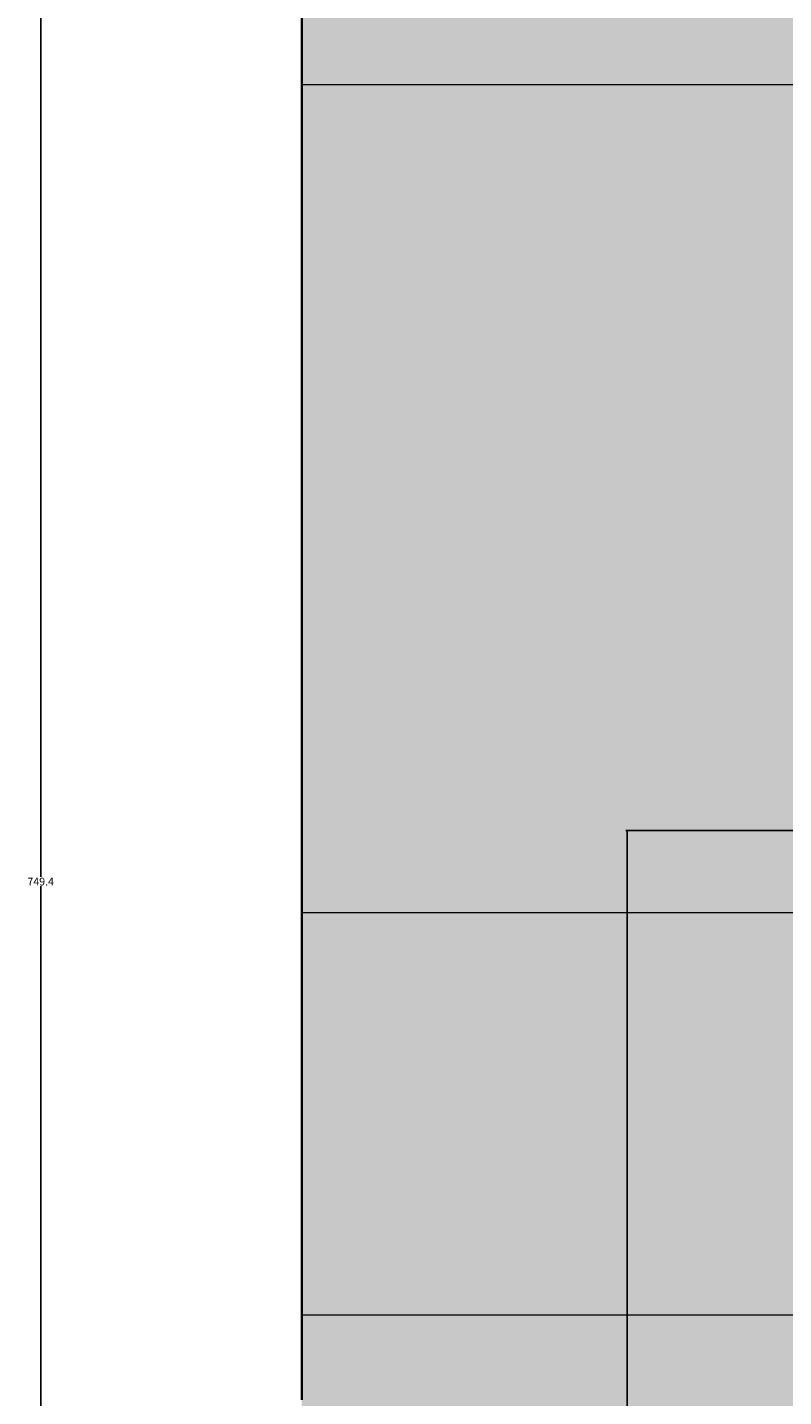
# Model space of a CAD drawing. Units: inches. Extents: x 8 to 634, y 41 to 867.
# Tile 5 of 21: x 8 to 117, y 380 to 577. Entities that reach past the tile are written whole.
import ezdxf

# ---------------------------------------------------------------- set-up
doc = ezdxf.new("R2010")
doc.units = ezdxf.units.IN
doc.header["$MEASUREMENT"] = 0
for name, color, linetype, lineweight in [('A-ANNO-DIMS', 2, 'Continuous', 18), ('A-WALL', 7, 'Continuous', 35), ('A-WALL-PANL', 7, 'Continuous', 18), ('A-WALL-PATT', 8, 'Continuous', 9)]:
    doc.layers.add(name, color=color, linetype=linetype, lineweight=lineweight)
doc.styles.get("Standard").update_dxf_attribs({"font": 'arial.ttf'})
doc.dimstyles.get("Standard").update_dxf_attribs({"dimtxt": 1.125, "dimasz": 0.18, "dimexe": 0.18, "dimexo": 0.0625, "dimgap": 0.09, "dimtad": 0, "dimtih": 1, "dimtoh": 1, "dimdec": 4, "dimzin": 0, "dimdsep": 46, "dimlunit": 4, "dimtxsty": 'Standard', "dimcen": 0.09, "dimadec": 0, "dimazin": 0, "dimtfac": 1, "dimtdec": 4, "dimtofl": 0, "dimtmove": 0, "dimatfit": 3, "dimfxl": 1, "dimtolj": 1, "dimtzin": 0, "dimarcsym": 0})

# ---------------------------------------------------------------- blocks, each defined once
blk = doc.blocks.new('*D20')
at = {"layer": 'A-ANNO-DIMS', "color": 0, "lineweight": -2, "transparency": 16777216}
for p, q in [((144.29, 828.98), (9.51, 828.98)), ((9.69, 828.8), (9.69, 454.93)), ((9.69, 79.74), (9.69, 453.6)), ((47.28, 79.56), (9.51, 79.56))]:
    blk.add_line(p, q, dxfattribs=at)
at = {"layer": 'A-ANNO-DIMS', "color": 0, "transparency": 16777216}
for points in [[(9.66, 828.8), (9.72, 828.8), (9.69, 828.98)], [(9.66, 79.74), (9.72, 79.74), (9.69, 79.56)]]:
    blk.add_solid(points, dxfattribs=at)
at = {"layer": 'Defpoints', "color": 0, "transparency": 16777216}
for p in [(9.69, 828.98), (144.36, 828.98), (47.34, 79.56)]:
    blk.add_point(p, dxfattribs=at)
at = {"layer": 'A-ANNO-DIMS', "color": 0, "transparency": 16777216, "insert": (9.69, 454.27), "char_height": 1.125, "attachment_point": 5}
blk.add_mtext('\\A1;749.4', dxfattribs=at)
blk = doc.blocks.new('*D43')
at = {"layer": 'A-ANNO-DIMS', "color": 0, "lineweight": -2, "transparency": 16777216}
for p, q in [((131.81, 461.65), (94.05, 461.65)), ((94.23, 461.47), (94.23, 373.6)), ((94.23, 284.42), (94.23, 372.29)), ((131.81, 284.24), (94.05, 284.24))]:
    blk.add_line(p, q, dxfattribs=at)
at = {"layer": 'A-ANNO-DIMS', "color": 0, "transparency": 16777216}
for points in [[(94.2, 461.47), (94.26, 461.47), (94.23, 461.65)], [(94.2, 284.42), (94.26, 284.42), (94.23, 284.24)]]:
    blk.add_solid(points, dxfattribs=at)
at = {"layer": 'Defpoints', "color": 0, "transparency": 16777216}
for p in [(94.23, 461.65), (131.88, 461.65), (131.88, 284.24)]:
    blk.add_point(p, dxfattribs=at)
at = {"layer": 'A-ANNO-DIMS', "color": 0, "transparency": 16777216, "insert": (94.23, 372.95), "char_height": 1.125, "attachment_point": 5}
blk.add_mtext('\\A1;177.4', dxfattribs=at)
blk = doc.blocks.new('*D58')
at = {"layer": 'A-ANNO-DIMS', "color": 0, "lineweight": -2, "transparency": 16777216}
for p, q in [((47.34, 569.23), (47.34, 607)), ((47.52, 606.82), (81.54, 606.82)), ((119.53, 606.82), (85.51, 606.82)), ((119.71, 569.23), (119.71, 607))]:
    blk.add_line(p, q, dxfattribs=at)
at = {"layer": 'A-ANNO-DIMS', "color": 0, "transparency": 16777216}
for points in [[(47.52, 606.85), (47.52, 606.79), (47.34, 606.82)], [(119.53, 606.85), (119.53, 606.79), (119.71, 606.82)]]:
    blk.add_solid(points, dxfattribs=at)
at = {"layer": 'Defpoints', "color": 0, "transparency": 16777216}
for p in [(119.71, 606.82), (47.34, 569.17), (119.71, 569.17)]:
    blk.add_point(p, dxfattribs=at)
at = {"layer": 'A-ANNO-DIMS', "color": 0, "transparency": 16777216, "insert": (83.52, 606.82), "char_height": 1.125, "attachment_point": 5}
blk.add_mtext('\\A1;72.37', dxfattribs=at)

msp = doc.modelspace()

# ---------------------------------------------------------------- hatches: boundary and pattern name
at = {"layer": 'A-WALL-PATT', "transparency": 33554687}
h = msp.add_hatch(dxfattribs=at)
h.set_pattern_fill('AR-CONC', color=256, scale=3.2)
h.paths.add_polyline_path([(119.7065, 697.6655), (47.3401, 697.6655), (47.3401, 569.1705), (119.7065, 569.1705)])
h.paths.add_polyline_path([(202.1558, 697.6655), (119.7065, 697.6655), (119.7065, 569.1705), (202.1558, 569.1705)])
h.paths.add_polyline_path([(284.6051, 697.6655), (202.1558, 697.6655), (202.1558, 569.1705), (284.6051, 569.1705)])
h.paths.add_polyline_path([(119.7065, 569.1705), (47.3401, 569.1705), (47.3401, 523.5555), (47.3401, 449.7533), (119.7065, 449.7533)])
h.paths.add_polyline_path([(342.6544, 682.1444), (360.785, 697.6655), (284.6051, 697.6655), (284.6051, 569.1705), (342.6544, 569.1705)])
h.paths.add_polyline_path([(342.6544, 569.1705), (284.6051, 569.1705), (284.6051, 449.7533), (342.6544, 449.7533)])
h.paths.add_polyline_path([(418.2881, 691.978), (418.2881, 697.6655), (360.785, 697.6655), (360.785, 569.1705), (418.2881, 569.1705)])
h.paths.add_polyline_path([(418.2881, 569.1705), (360.785, 569.1705), (360.785, 523.5555), (360.785, 449.7533), (418.2881, 449.7533)])
h.paths.add_polyline_path([(594.3501, 697.6655), (539.0002, 697.6655), (539.0002, 691.978), (539.0002, 569.1705), (594.3501, 569.1705)])
h.paths.add_polyline_path([(594.3501, 523.5555), (594.3501, 569.1705), (539.0002, 569.1705), (539.0002, 451.6305), (594.3501, 451.6305)])
h.paths.add_polyline_path([(594.3501, 451.6305), (539.0002, 451.6305), (539.0002, 391.7598), (594.3501, 391.7598)])
h.paths.add_polyline_path([(594.3501, 391.7598), (539.0002, 391.7598), (539.0002, 276.166), (594.3501, 276.166)])
h.paths.add_polyline_path([(418.2881, 449.7533), (360.785, 449.7533), (360.785, 391.7598), (418.2881, 391.7598)])
h.paths.add_polyline_path([(342.6544, 449.7533), (284.6051, 449.7533), (284.6051, 391.7598), (342.6544, 391.7598)])
h.paths.add_polyline_path([(342.6544, 391.7598), (284.6051, 391.7598), (284.6051, 272.3426), (342.6544, 272.3426)])
h.paths.add_polyline_path([(418.2881, 391.7598), (360.785, 391.7598), (360.785, 272.3426), (418.2881, 272.3426)])
h.paths.add_polyline_path([(418.2881, 272.3426), (360.785, 272.3426), (360.785, 235.5555), (418.2881, 235.5555)])
h.paths.add_polyline_path([(342.6544, 272.3426), (284.6051, 272.3426), (284.6051, 235.5555), (295.0049, 235.5555), (342.6544, 235.5555)])
h.paths.add_polyline_path([(594.3501, 276.166), (539.0002, 276.166), (539.0002, 228.4951), (594.3501, 228.4951)])
h.paths.add_polyline_path([(594.3501, 228.4951), (539.0002, 228.4951), (539.0002, 91.5417), (594.3501, 91.5417)])
h.paths.add_polyline_path([(418.2881, 235.5555), (360.785, 235.5555), (360.785, 91.5417), (418.2881, 91.5417)])
h.paths.add_polyline_path([(284.6051, 272.3426), (119.7065, 272.3426), (119.7065, 235.5555), (284.6051, 235.5555)])
h.paths.add_polyline_path([(119.7065, 272.3426), (47.3401, 272.3426), (47.3401, 235.5555), (47.3401, 91.5555), (63.5448, 91.5555), (63.5448, 227.8036), (268.998, 227.8036), (268.998, 91.5555), (295.0049, 91.5555), (295.0049, 222.583), (271.9787, 222.583), (271.9787, 229.0481), (62.4019, 229.0481), (62.4019, 222.583), (61.1827, 222.583), (61.1827, 235.5555), (119.7065, 235.5555)])
h.paths.add_polyline_path([(119.7065, 391.7598), (47.3401, 391.7598), (47.3401, 379.5555), (47.3401, 272.3426), (119.7065, 272.3426)])
h.paths.add_polyline_path([(119.7065, 449.7533), (47.3401, 449.7533), (47.3401, 391.7598), (119.7065, 391.7598)])
h.paths.add_polyline_path([(202.1558, 449.7533), (119.7065, 449.7533), (119.7065, 391.7598), (202.1558, 391.7598)])
h.paths.add_polyline_path([(284.6051, 449.7533), (202.1558, 449.7533), (202.1558, 391.7598), (284.6051, 391.7598)])

# ---------------------------------------------------------------- linework, layer by layer
at = {"layer": 'A-WALL'}
for p, q in [((47.3401, 523.5555), (47.3401, 697.6655)), ((47.3401, 379.5555), (47.3401, 523.5555))]:
    msp.add_line(p, q, dxfattribs=at)
at = {"layer": 'A-WALL-PANL'}
for p, q in [((418.2881, 569.1705), (47.3401, 569.1705)), ((119.7065, 449.7533), (47.3401, 449.7533)), ((418.2881, 391.7598), (47.3401, 391.7598))]:
    msp.add_line(p, q, dxfattribs=at)

# ---------------------------------------------------------------- dimensions: what is measured, and where the dimension line sits
at = {"layer": 'A-ANNO-DIMS'}
for base, p1, p2, picture, middle in [((9.6901, 828.9821), (47.3401, 79.5555), (144.3564, 828.9821), '*D20', (9.6901, 454.2688)), ((94.2271, 461.6505), (131.8771, 284.2398), (131.8771, 461.6505), '*D43', (94.2271, 372.9452))]:
    dim = msp.add_linear_dim(base=base, p1=p1, p2=p2, angle=90, dimstyle='Standard', override={"dimdec": 1, "dimlfac": 1, "dimrnd": 0, "dimzin": 0, "dimdsep": 46, "dimlunit": 2}, dxfattribs=at)
    dim.commit()
    dim.dimension.update_dxf_attribs({"geometry": picture, "text_midpoint": middle})
dim = msp.add_linear_dim(base=(119.7065, 606.8205), p1=(47.3401, 569.1705), p2=(119.7065, 569.1705), dimstyle='Standard', override={"dimdec": 2, "dimlfac": 1, "dimrnd": 0, "dimzin": 0, "dimdsep": 46, "dimlunit": 2}, dxfattribs=at)
dim.commit()
dim.dimension.update_dxf_attribs({"geometry": '*D58', "text_midpoint": (83.5233, 606.8205)})

doc.saveas('drawing.dxf')
